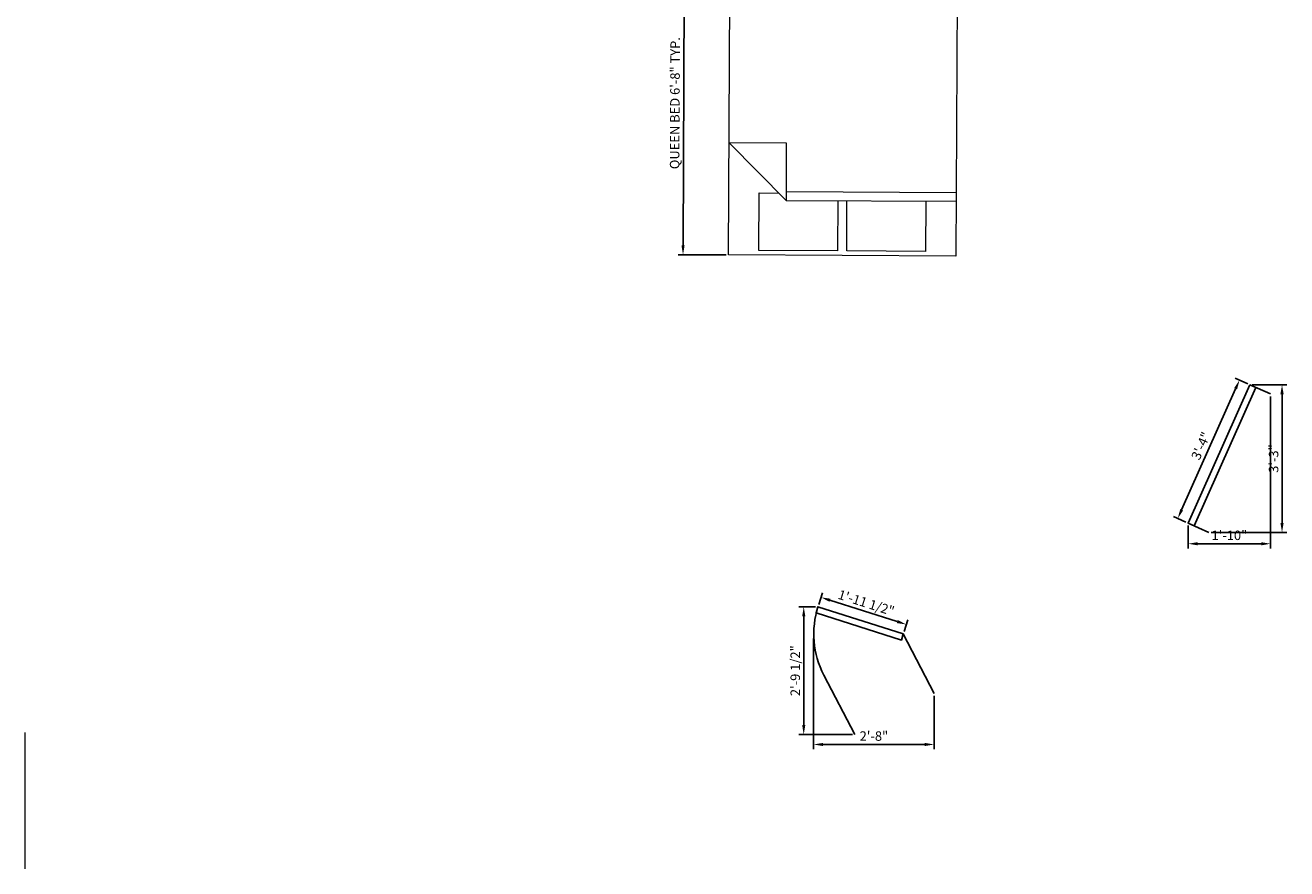
# Model space of a CAD drawing. Units: inches. Extents: x -2945 to -2182, y 3541 to 4172.
# Tile 1 of 5: x -2945 to -2612, y 3678 to 3900. Entities that reach past the tile are written whole.
import ezdxf

# ---------------------------------------------------------------- set-up
doc = ezdxf.new("R2010")
doc.units = ezdxf.units.IN
for name, color, linetype, lineweight in [('A-ANNO-DIMS', 2, 'Continuous', 18), ('A-DOOR', 3, 'Continuous', 25), ('A-FURN', 9, 'Continuous', 18), ('A-REFR', 8, 'Continuous', 13)]:
    doc.layers.add(name, color=color, linetype=linetype, lineweight=lineweight)
doc.styles.get("Standard").update_dxf_attribs({"font": 'arial.ttf'})
doc.dimstyles.new('ISO-25', dxfattribs={"dimtxt": 2.5, "dimasz": 2.5, "dimexe": 1.25, "dimexo": 0.625, "dimtad": 1, "dimdec": 0, "dimlunit": 3, "dimtxsty": 'Standard', "dimcen": 2.5, "dimadec": 0, "dimazin": 0, "dimtfac": 1, "dimtdec": 0, "dimtmove": 0, "dimatfit": 3, "dimfxl": 1, "dimarcsym": 0})

# ---------------------------------------------------------------- blocks, each defined once
blk = doc.blocks.new('Bed - Queen')
for p, q in [((0, -80.00003), (0, 0)), ((0, 0), (59.99999, 0)), ((59.99999, 0), (59.99999, -80.00003)), ((7.99999, -1.2), (28.79998, -1.2)), ((7.99999, -14.4), (7.99999, -1.2)), ((28.79998, -1.2), (28.79998, -14.4)), ((31.19999, -1.2), (51.99999, -1.2)), ((31.19999, -14.4), (31.19999, -1.2)), ((51.99999, -1.2), (51.99999, -16.4)), ((0, -14.4), (44.8, -14.4)), ((59.99999, -29.6), (44.8, -14.4)), ((44.8, -14.4), (44.8, -29.6)), ((51.99999, -16.4), (46.79936, -16.4)), ((44.8, -16.8), (0, -16.8)), ((44.8, -29.6), (59.99999, -29.6)), ((59.99999, -80.00003), (0, -80.00003))]:
    blk.add_line(p, q)
blk = doc.blocks.new('*U3')
for p, q in [((0, 0), (0, 6)), ((40, 0), (40, 6))]:
    blk.add_line(p, q)
blk.add_lwpolyline([(0, 0), (40, 0), (40, 1.75), (0, 1.75)], close=True)
blk = doc.blocks.new('*U6')
for p, q in [((-600, 0), (-600, -450)), ((0, 0), (0, -450))]:
    blk.add_line(p, q)
blk.add_lwpolyline([(0, 0), (-424.3, 424.3), (-455.2, 393.3), (-30.9, -30.9)], close=True)
blk.add_arc((0, 0), 600, 135, 180)
blk = doc.blocks.new('*D12')
at = {"layer": 'A-ANNO-DIMS', "color": 0, "lineweight": -2, "transparency": 16777216}
for p, q in [((-2759.27, 3919.61), (-2771.89, 3919.67)), ((-2770.65, 3917.16), (-2770.99, 3842.16)), ((-2759.63, 3839.61), (-2772.25, 3839.67))]:
    blk.add_line(p, q, dxfattribs=at)
at = {"layer": 'A-ANNO-DIMS', "color": 0, "transparency": 16777216}
for points in [[(-2771.07, 3917.16), (-2770.23, 3917.16), (-2770.64, 3919.66)], [(-2771.41, 3842.16), (-2770.58, 3842.16), (-2771, 3839.66)]]:
    blk.add_solid(points, dxfattribs=at)
at = {"layer": 'Defpoints', "color": 0, "transparency": 16777216}
for p in [(-2758.64, 3919.61), (-2771, 3839.66), (-2759, 3839.61)]:
    blk.add_point(p, dxfattribs=at)
at = {"layer": 'A-ANNO-DIMS', "color": 0, "transparency": 16777216, "insert": (-2772.82, 3879.67), "char_height": 2.5, "attachment_point": 5, "rotation": 89.7398}
blk.add_mtext('QUEEN BED 6\'-8" TYP.', dxfattribs=at)
blk = doc.blocks.new('*D71')
at = {"layer": 'A-ANNO-DIMS', "color": 0, "lineweight": -2, "transparency": 16777216}
for p, q in [((-2621.99, 3805.63), (-2625.3, 3807.1)), ((-2639.43, 3772.35), (-2625.18, 3804.31)), ((-2638.28, 3769.09), (-2641.59, 3770.57))]:
    blk.add_line(p, q, dxfattribs=at)
at = {"layer": 'A-ANNO-DIMS', "color": 0, "transparency": 16777216}
for points in [[(-2625.56, 3804.48), (-2624.8, 3804.14), (-2624.16, 3806.59)], [(-2639.81, 3772.52), (-2639.05, 3772.18), (-2640.45, 3770.06)]]:
    blk.add_solid(points, dxfattribs=at)
at = {"layer": 'Defpoints', "color": 0, "transparency": 16777216}
for p in [(-2624.16, 3806.59), (-2621.42, 3805.37), (-2637.71, 3768.84)]:
    blk.add_point(p, dxfattribs=at)
at = {"layer": 'A-ANNO-DIMS', "color": 0, "transparency": 16777216, "insert": (-2634.04, 3789.1), "char_height": 2.5, "attachment_point": 5, "rotation": 65.9615}
blk.add_mtext('3\'-4"', dxfattribs=at)
blk = doc.blocks.new('*D72')
at = {"layer": 'A-ANNO-DIMS', "color": 0, "lineweight": -2, "transparency": 16777216}
for p, q in [((-2615.94, 3802.3), (-2615.94, 3762.15)), ((-2637.71, 3768.22), (-2637.71, 3762.15)), ((-2635.21, 3763.4), (-2618.44, 3763.4))]:
    blk.add_line(p, q, dxfattribs=at)
at = {"layer": 'A-ANNO-DIMS', "color": 0, "transparency": 16777216}
for points in [[(-2635.21, 3763.81), (-2635.21, 3762.98), (-2637.71, 3763.4)], [(-2618.44, 3763.81), (-2618.44, 3762.98), (-2615.94, 3763.4)]]:
    blk.add_solid(points, dxfattribs=at)
at = {"layer": 'Defpoints', "color": 0, "transparency": 16777216}
for p in [(-2615.94, 3802.93), (-2637.71, 3768.84), (-2615.94, 3763.4)]:
    blk.add_point(p, dxfattribs=at)
at = {"layer": 'A-ANNO-DIMS', "color": 0, "transparency": 16777216, "insert": (-2626.83, 3765.3), "char_height": 2.5, "attachment_point": 5}
blk.add_mtext('1\'-10"', dxfattribs=at)
blk = doc.blocks.new('*D73')
at = {"layer": 'A-ANNO-DIMS', "color": 0, "lineweight": -2, "transparency": 16777216}
for p, q in [((-2620.79, 3805.37), (-2611.69, 3805.37)), ((-2612.94, 3768.9), (-2612.94, 3802.87)), ((-2631.61, 3766.4), (-2611.69, 3766.4))]:
    blk.add_line(p, q, dxfattribs=at)
at = {"layer": 'A-ANNO-DIMS', "color": 0, "transparency": 16777216}
for points in [[(-2613.36, 3802.87), (-2612.52, 3802.87), (-2612.94, 3805.37)], [(-2613.36, 3768.9), (-2612.52, 3768.9), (-2612.94, 3766.4)]]:
    blk.add_solid(points, dxfattribs=at)
at = {"layer": 'Defpoints', "color": 0, "transparency": 16777216}
for p in [(-2621.42, 3805.37), (-2612.94, 3805.37), (-2632.23, 3766.4)]:
    blk.add_point(p, dxfattribs=at)
at = {"layer": 'A-ANNO-DIMS', "color": 0, "transparency": 16777216, "insert": (-2614.84, 3785.88), "char_height": 2.5, "attachment_point": 5, "rotation": 90}
blk.add_mtext('3\'-3"', dxfattribs=at)
blk = doc.blocks.new('*D74')
at = {"layer": 'A-ANNO-DIMS', "color": 0, "lineweight": -2, "transparency": 16777216}
for p, q in [((-2735.2, 3747.37), (-2734.22, 3750.44)), ((-2732.22, 3748.49), (-2714.47, 3742.86)), ((-2712.68, 3740.22), (-2711.7, 3743.3))]:
    blk.add_line(p, q, dxfattribs=at)
at = {"layer": 'A-ANNO-DIMS', "color": 0, "transparency": 16777216}
for points in [[(-2732.09, 3748.89), (-2732.34, 3748.1), (-2734.6, 3749.25)], [(-2714.34, 3743.26), (-2714.59, 3742.46), (-2712.08, 3742.1)]]:
    blk.add_solid(points, dxfattribs=at)
at = {"layer": 'Defpoints', "color": 0, "transparency": 16777216}
for p in [(-2735.38, 3746.77), (-2712.08, 3742.1), (-2712.87, 3739.63)]:
    blk.add_point(p, dxfattribs=at)
at = {"layer": 'A-ANNO-DIMS', "color": 0, "transparency": 16777216, "insert": (-2722.76, 3747.51), "char_height": 2.5, "attachment_point": 5, "rotation": 342.3931}
blk.add_mtext('1\'-11 1/2"', dxfattribs=at)
blk = doc.blocks.new('*D75')
at = {"layer": 'A-ANNO-DIMS', "color": 0, "lineweight": -2, "transparency": 16777216}
for p, q in [((-2736.01, 3746.77), (-2740.4, 3746.77)), ((-2739.15, 3744.27), (-2739.15, 3715.53)), ((-2726.32, 3713.03), (-2740.4, 3713.03))]:
    blk.add_line(p, q, dxfattribs=at)
at = {"layer": 'A-ANNO-DIMS', "color": 0, "transparency": 16777216}
for points in [[(-2739.56, 3744.27), (-2738.73, 3744.27), (-2739.15, 3746.77)], [(-2739.56, 3715.53), (-2738.73, 3715.53), (-2739.15, 3713.03)]]:
    blk.add_solid(points, dxfattribs=at)
at = {"layer": 'Defpoints', "color": 0, "transparency": 16777216}
for p in [(-2735.38, 3746.77), (-2739.15, 3713.03), (-2725.69, 3713.03)]:
    blk.add_point(p, dxfattribs=at)
at = {"layer": 'A-ANNO-DIMS', "color": 0, "transparency": 16777216, "insert": (-2741.06, 3729.9), "char_height": 2.5, "attachment_point": 5, "rotation": 90}
blk.add_mtext('2\'-9 1/2"', dxfattribs=at)
blk = doc.blocks.new('*D76')
at = {"layer": 'A-ANNO-DIMS', "color": 0, "lineweight": -2, "transparency": 16777216}
for p, q in [((-2736.55, 3738.36), (-2736.55, 3709.18)), ((-2704.72, 3723.27), (-2704.72, 3709.18)), ((-2734.05, 3710.43), (-2707.22, 3710.43))]:
    blk.add_line(p, q, dxfattribs=at)
at = {"layer": 'A-ANNO-DIMS', "color": 0, "transparency": 16777216}
for points in [[(-2734.05, 3710.84), (-2734.05, 3710.01), (-2736.55, 3710.43)], [(-2707.22, 3710.84), (-2707.22, 3710.01), (-2704.72, 3710.43)]]:
    blk.add_solid(points, dxfattribs=at)
at = {"layer": 'Defpoints', "color": 0, "transparency": 16777216}
for p in [(-2736.55, 3738.98), (-2704.72, 3723.9), (-2704.72, 3710.43)]:
    blk.add_point(p, dxfattribs=at)
at = {"layer": 'A-ANNO-DIMS', "color": 0, "transparency": 16777216, "insert": (-2720.63, 3712.33), "char_height": 2.5, "attachment_point": 5}
blk.add_mtext('2\'-8"', dxfattribs=at)

msp = doc.modelspace()

# ---------------------------------------------------------------- linework, layer by layer
at = {"layer": 'A-REFR'}
msp.add_line((-2944.57, 3677.63), (-2944.57, 3713.63), dxfattribs=at)

# ---------------------------------------------------------------- block references
at = {"layer": 'A-DOOR', "rotation": 245.961546287805}
msp.add_blockref('*U3', (-2621.42, 3805.37), dxfattribs=at)
at = {"layer": 'A-DOOR', "xscale": 0.0393700787401575, "yscale": 0.0393700787401575, "zscale": 0.0393700787401575, "rotation": 27.39306522065776}
msp.add_blockref('*U6', (-2712.87, 3739.63), dxfattribs=at)
at = {"layer": 'A-FURN', "rotation": 179.7397650528711}
msp.add_blockref('Bed - Queen', (-2699, 3839.33), dxfattribs=at)

# ---------------------------------------------------------------- dimensions: what is measured, and where the dimension line sits
at = {"layer": 'A-ANNO-DIMS'}
dim = msp.add_linear_dim(base=(-2771, 3839.66), p1=(-2758.64, 3919.61), p2=(-2759, 3839.61), angle=269.7398, text='QUEEN BED <> TYP.', dimstyle='ISO-25', override={"dimdec": 1, "dimlfac": 1, "dimrnd": 0, "dimzin": 1, "dimdsep": 46, "dimlunit": 4, "dimfrac": 2}, dxfattribs=at)
dim.commit()
dim.dimension.update_dxf_attribs({"geometry": '*D12', "text_midpoint": (-2772.82, 3879.67)})
for base, p1, p2, angle, picture, middle in [((-2624.16, 3806.59), (-2637.71, 3768.84), (-2621.42, 3805.37), 65.9615, '*D71', (-2634.04, 3789.1)), ((-2612.94, 3805.37), (-2632.23, 3766.4), (-2621.42, 3805.37), 90, '*D73', (-2614.84, 3785.88)), ((-2712.08, 3742.1), (-2735.38, 3746.77), (-2712.87, 3739.63), 342.3931, '*D74', (-2722.76, 3747.51)), ((-2739.15, 3713.03), (-2735.38, 3746.77), (-2725.69, 3713.03), 90, '*D75', (-2741.06, 3729.9))]:
    dim = msp.add_linear_dim(base=base, p1=p1, p2=p2, angle=angle, dimstyle='ISO-25', override={"dimdec": 1, "dimlfac": 1, "dimrnd": 0, "dimzin": 1, "dimdsep": 46, "dimlunit": 4, "dimfrac": 2}, dxfattribs=at)
    dim.commit()
    dim.dimension.update_dxf_attribs({"geometry": picture, "text_midpoint": middle})
for base, p1, p2, picture, middle in [((-2615.94, 3763.4), (-2637.71, 3768.84), (-2615.94, 3802.93), '*D72', (-2626.83, 3765.3)), ((-2704.72, 3710.43), (-2736.55, 3738.98), (-2704.72, 3723.9), '*D76', (-2720.63, 3712.33))]:
    dim = msp.add_linear_dim(base=base, p1=p1, p2=p2, dimstyle='ISO-25', override={"dimdec": 1, "dimlfac": 1, "dimrnd": 0, "dimzin": 1, "dimdsep": 46, "dimlunit": 4, "dimfrac": 2}, dxfattribs=at)
    dim.commit()
    dim.dimension.update_dxf_attribs({"geometry": picture, "text_midpoint": middle})

doc.saveas('drawing.dxf')
